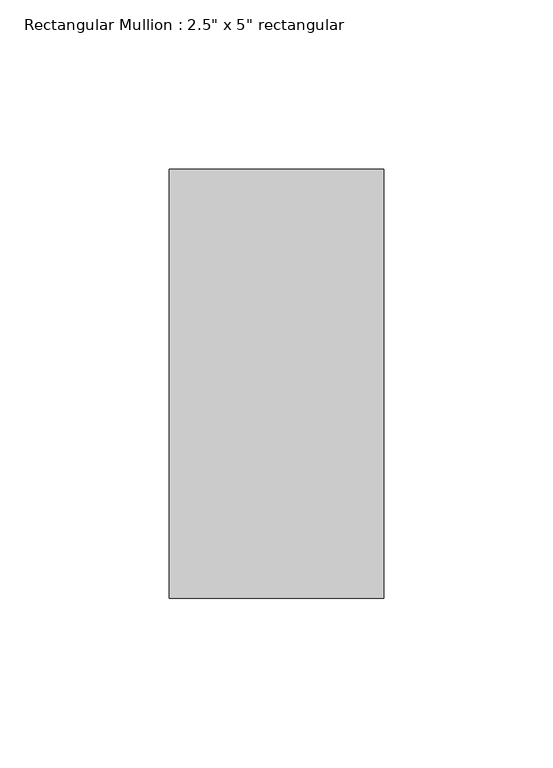
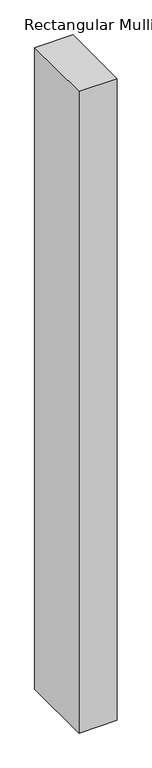
"""IFC4 building model written with IfcOpenShell, lengths in millimetres: member geometry."""

from ifc_helpers import new_model, si_unit, frame, origin, place, context, project, spatial, polyline, outline, extrude, source, transform, mapped, element, save


def member_62e0d4bf(model_context):
    return source(origin(), model_context, "Body", "SweptSolid", [
        extrude(outline(polyline([(0.0, 63.5), (0.0, -63.5), (-63.5, -63.5), (-63.5, 63.5), (0.0, 63.5)])), frame((0.0, 0.0, -1126.7437105), z_axis=(0.0, 0.0, 1.0), x_axis=(1.0, 0.0, 0.0)), (0.0, 0.0, 1.0), 1126.7437105),
    ])


if __name__ == "__main__":
    model = new_model("IFC4")
    model_context = context("Model", 3, world=origin())
    ifc_project = project(units=[si_unit("LENGTHUNIT", "METRE", prefix="MILLI")], contexts=[model_context])
    site = spatial("IfcSite", under=ifc_project)
    building = spatial("IfcBuilding", under=site)
    placement = place(None, origin())
    member_shape = member_62e0d4bf(model_context)
    element("IfcMember", 1, ObjectType="Rectangular Mullion : 2.5\" x 5\" rectangular", at=placement, inside=building, context=model_context, shape_type="MappedRepresentation", body=[
        mapped(member_shape, transform((0.0, 0.0, 0.0), x_axis=(1.0, 0.0, 0.0), y_axis=(0.0, 1.0, 0.0), z_axis=(0.0, 0.0, 1.0))),
    ])
    save(model, "model.ifc")

# Revit data of these elements
# Type "Rectangular Mullion : 2.5\" x 5\" rectangular"
#   built-in parameter 1007304 = 0.416667 (stored number, unit not read)
#   built-in parameter 1007301 = 0.104167 (stored number, unit not read)
#   built-in parameter 1007300 = 0.104167 (stored number, unit not read)
# Element 1 (IfcMember, "Rectangular Mullion : 2.5\" x 5\" rectangular")
#   Materials on its faces: "Aluminum"
# Materials
#   "Aluminum": class "Metal", colour RGB 247 247 247, transparency 0, Description = "Aluminum 6061", Cost = 0
